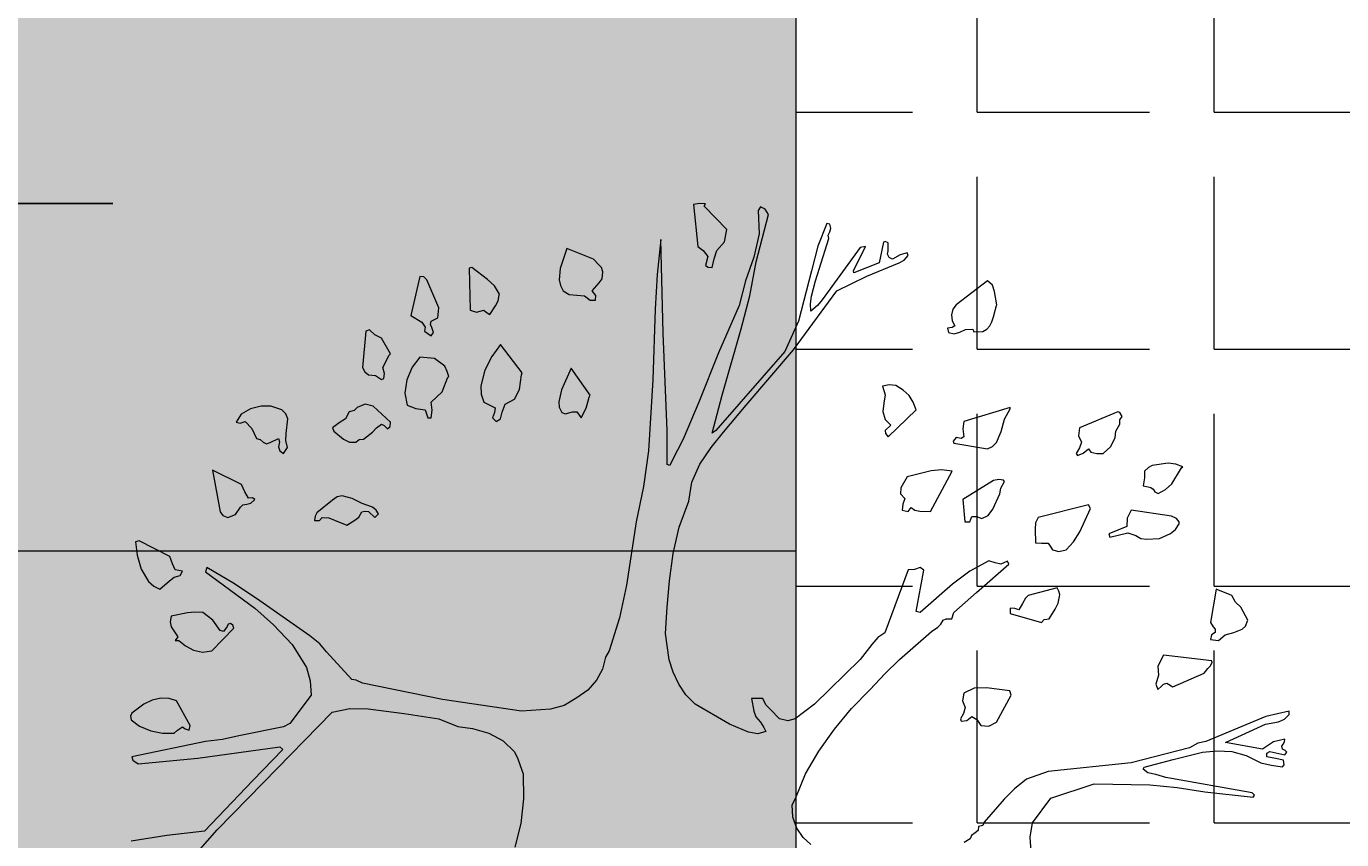
# Model space of a CAD drawing. Units: inches. Extents: x 84 to 1044, y -280 to 906.
# Tile 12 of 105: x 482 to 521, y -49 to -25. Entities that reach past the tile are written whole.
import ezdxf

# ---------------------------------------------------------------- set-up
doc = ezdxf.new("R2010")
doc.units = ezdxf.units.IN
for name, color, linetype, lineweight in [('A-ANNO-DIMS', 2, 'Continuous', 18), ('L-HRDS', 32, 'Continuous', 18), ('L-PLNT', 114, 'Continuous', 15)]:
    doc.layers.add(name, color=color, linetype=linetype, lineweight=lineweight)
doc.layers.add('L-HRDS-PATT', color=23, linetype='Continuous', lineweight=9, true_color=0xc2877b)
doc.layers.add('L-PLNT-PATT', color=9, linetype='Continuous', lineweight=9, true_color=0xafd9aa)
doc.styles.get("Standard").update_dxf_attribs({"font": 'arial.ttf'})
doc.dimstyles.get("Standard").update_dxf_attribs({"dimtxt": 0.18, "dimasz": 0.18, "dimexe": 0.18, "dimexo": 0.0625, "dimgap": 0.09, "dimtad": 0, "dimtih": 1, "dimtoh": 1, "dimdec": 4, "dimzin": 0, "dimdsep": 46, "dimtxsty": 'Standard', "dimcen": 0.09, "dimadec": 0, "dimazin": 0, "dimtfac": 1, "dimtdec": 4, "dimtofl": 0, "dimtmove": 0, "dimatfit": 3, "dimfxl": 1, "dimtolj": 1, "dimtzin": 0, "dimarcsym": 0})

# ---------------------------------------------------------------- blocks, each defined once
blk = doc.blocks.new('A$C37E508DF')
for p, q in [((0.6329, 1.5111), (0.6367, 1.5175)), ((0.6475, 1.4545), (0.6329, 1.5111)), ((0.6367, 1.5175), (0.6423, 1.5201)), ((0.6423, 1.5201), (0.6453, 1.5158)), ((0.6453, 1.5158), (0.644, 1.4879)), ((0.6826, 1.493), (0.7096, 1.5209)), ((0.7083, 1.5239), (0.7152, 1.5244)), ((0.7096, 1.5209), (0.7083, 1.5239)), ((0.7152, 1.5244), (0.7225, 1.5231)), ((0.7225, 1.5231), (0.7174, 1.4729)), ((0.5583, 1.4948), (0.5596, 1.4995)), ((0.5596, 1.4905), (0.5583, 1.4948)), ((0.5596, 1.4995), (0.563, 1.5003)), ((0.563, 1.5003), (0.5737, 1.4733)), ((0.4897, 1.4772), (0.4935, 1.4789)), ((0.4935, 1.4789), (0.4952, 1.478)), ((0.5613, 1.4862), (0.5596, 1.4905)), ((0.5608, 1.4823), (0.5613, 1.4862)), ((0.5767, 1.4317), (0.5608, 1.4823)), ((0.644, 1.4879), (0.6505, 1.46)), ((0.6852, 1.4785), (0.6826, 1.493)), ((0.6946, 1.4682), (0.6852, 1.4785)), ((0.7589, 1.3691), (0.7615, 1.481)), ((0.7615, 1.481), (0.7658, 1.4395)), ((0.4657, 1.4622), (0.4669, 1.4652)), ((0.4669, 1.4652), (0.4755, 1.463)), ((0.4755, 1.463), (0.4845, 1.4575)), ((0.4884, 1.4596), (0.4905, 1.4635)), ((0.4897, 1.4678), (0.4897, 1.4772)), ((0.4905, 1.4635), (0.4897, 1.4678)), ((0.4952, 1.478), (0.5004, 1.4532)), ((0.5313, 1.4437), (0.5167, 1.4729)), ((0.5167, 1.4729), (0.5231, 1.4716)), ((0.5231, 1.4716), (0.5686, 1.409)), ((0.5737, 1.4733), (0.5814, 1.4437)), ((0.6976, 1.4579), (0.6946, 1.4682)), ((0.7109, 1.4682), (0.7053, 1.4609)), ((0.7174, 1.4729), (0.7109, 1.4682)), ((0.8421, 1.4575), (0.8739, 1.4703)), ((0.8739, 1.4703), (0.882, 1.4463)), ((0.4708, 1.4566), (0.4657, 1.4622)), ((0.4764, 1.4532), (0.4708, 1.4566)), ((0.5154, 1.4373), (0.4764, 1.4532)), ((0.4845, 1.4575), (0.4884, 1.4596)), ((0.5004, 1.4532), (0.5308, 1.4412)), ((0.6552, 1.4137), (0.6475, 1.4545)), ((0.6505, 1.46), (0.6603, 1.4317)), ((0.7002, 1.4476), (0.6976, 1.4579)), ((0.7049, 1.448), (0.7002, 1.4476)), ((0.7083, 1.4502), (0.7049, 1.448)), ((0.7053, 1.4609), (0.7083, 1.4502)), ((0.831, 1.4424), (0.8323, 1.4476)), ((0.8323, 1.4476), (0.8357, 1.451)), ((0.8357, 1.451), (0.8421, 1.4575)), ((0.9686, 1.4334), (0.9875, 1.4476)), ((0.9875, 1.4476), (0.9905, 1.4467)), ((0.9905, 1.4467), (0.9896, 1.3966)), ((0.3649, 1.4266), (0.3709, 1.4317)), ((0.3709, 1.4317), (0.4086, 1.403)), ((0.551, 1.4197), (0.5154, 1.4373)), ((0.5308, 1.4412), (0.5313, 1.4437)), ((0.5814, 1.4133), (0.5767, 1.4317)), ((0.5814, 1.4437), (0.5969, 1.3833)), ((0.6603, 1.4317), (0.668, 1.4021)), ((0.7658, 1.4395), (0.7684, 1.3979)), ((0.8318, 1.4343), (0.831, 1.4424)), ((0.8353, 1.4292), (0.8318, 1.4343)), ((0.8829, 1.433), (0.8816, 1.4262)), ((0.882, 1.4463), (0.8829, 1.433)), ((0.9605, 1.4257), (0.9686, 1.4334)), ((1.0269, 1.3996), (1.0411, 1.433)), ((1.0411, 1.433), (1.045, 1.4365)), ((1.045, 1.4365), (1.0497, 1.4369)), ((1.0497, 1.4369), (1.0604, 1.3901)), ((0.3598, 1.403), (0.3628, 1.4189)), ((0.3628, 1.4189), (0.3649, 1.4266)), ((0.6029, 1.3494), (0.551, 1.4197)), ((0.8434, 1.4197), (0.8353, 1.4292)), ((0.8391, 1.4141), (0.8434, 1.4197)), ((0.8709, 1.4154), (0.8619, 1.4146)), ((0.8781, 1.4197), (0.8709, 1.4154)), ((0.8816, 1.4262), (0.8781, 1.4197)), ((0.9545, 1.4159), (0.9605, 1.4257)), ((0.9549, 1.4146), (0.9545, 1.4159)), ((0.3602, 1.4021), (0.3598, 1.403)), ((0.364, 1.3888), (0.3602, 1.4021)), ((0.4086, 1.403), (0.4125, 1.3979)), ((0.5686, 1.409), (0.5741, 1.4021)), ((0.5741, 1.4021), (0.5823, 1.3953)), ((0.5827, 1.4043), (0.5814, 1.4133)), ((0.5823, 1.3953), (0.5827, 1.4043)), ((0.6655, 1.3743), (0.6552, 1.4137)), ((0.668, 1.4021), (0.6925, 1.3455)), ((0.8395, 1.4086), (0.8391, 1.4141)), ((0.846, 1.4086), (0.8395, 1.4086)), ((0.8528, 1.4137), (0.846, 1.4086)), ((0.8619, 1.4146), (0.8528, 1.4137)), ((0.9558, 1.4077), (0.9549, 1.4146)), ((0.9592, 1.4017), (0.9558, 1.4077)), ((0.966, 1.3914), (0.9592, 1.4017)), ((1.0282, 1.3876), (1.0269, 1.3996)), ((0.3657, 1.3828), (0.364, 1.3888)), ((0.4125, 1.3979), (0.4142, 1.391)), ((0.4142, 1.391), (0.4134, 1.3837)), ((0.7684, 1.3979), (0.771, 1.3134)), ((0.9703, 1.3944), (0.966, 1.3914)), ((0.9733, 1.3966), (0.9703, 1.3944)), ((0.9819, 1.3944), (0.9733, 1.3966)), ((0.9896, 1.3966), (0.9819, 1.3944)), ((1.0359, 1.3833), (1.0282, 1.3876)), ((1.0604, 1.3901), (1.0471, 1.3824)), ((0.3683, 1.3781), (0.3657, 1.3828)), ((0.3718, 1.3738), (0.3683, 1.3781)), ((0.3765, 1.3713), (0.3718, 1.3738)), ((0.3872, 1.3708), (0.3765, 1.3713)), ((0.3885, 1.3738), (0.3872, 1.3708)), ((0.3971, 1.3734), (0.3885, 1.3738)), ((0.4039, 1.3704), (0.3971, 1.3734)), ((0.4108, 1.3683), (0.4039, 1.3704)), ((0.4134, 1.3837), (0.4099, 1.3781)), ((0.4099, 1.3781), (0.4134, 1.376)), ((0.4176, 1.37), (0.4108, 1.3683)), ((0.4134, 1.376), (0.4189, 1.3751)), ((0.4189, 1.3751), (0.4176, 1.37)), ((0.5969, 1.3833), (0.6132, 1.3472)), ((0.6882, 1.2949), (0.6655, 1.3743)), ((0.7538, 1.2529), (0.7589, 1.3691)), ((1.0334, 1.37), (1.0351, 1.376)), ((1.0359, 1.3661), (1.0334, 1.37)), ((1.0351, 1.376), (1.0368, 1.3794)), ((1.0368, 1.3794), (1.0359, 1.3833)), ((1.0441, 1.3717), (1.0359, 1.3661)), ((1.0471, 1.3824), (1.0432, 1.3764)), ((1.0432, 1.3764), (1.0441, 1.3717)), ((1.1033, 1.367), (1.1097, 1.373)), ((1.1097, 1.373), (1.114, 1.3717)), ((1.114, 1.3717), (1.1183, 1.328)), ((0.9274, 1.3215), (0.9532, 1.3554)), ((0.9532, 1.3554), (0.9635, 1.3413)), ((1.0848, 1.3443), (1.0955, 1.3631)), ((1.0955, 1.3631), (1.1033, 1.367)), ((0.6595, 1.2829), (0.6029, 1.3494)), ((0.6132, 1.3472), (0.6959, 1.2529)), ((0.6925, 1.3455), (0.7161, 1.2868)), ((0.9635, 1.3413), (0.9721, 1.325)), ((1.0197, 1.3297), (1.0321, 1.3387)), ((1.0321, 1.3387), (1.0497, 1.3404)), ((1.0497, 1.3404), (1.0587, 1.3284)), ((1.0861, 1.343), (1.0848, 1.3443)), ((1.0938, 1.328), (1.0861, 1.343)), ((0.846, 1.2949), (0.8687, 1.3271)), ((0.8687, 1.3271), (0.8803, 1.3014)), ((0.9279, 1.3194), (0.9274, 1.3215)), ((0.9721, 1.325), (0.9768, 1.3061)), ((1.0149, 1.3172), (1.0171, 1.3232)), ((1.0171, 1.3232), (1.0197, 1.3297)), ((1.0587, 1.3284), (1.0651, 1.3134)), ((1.0917, 1.3207), (1.0938, 1.328)), ((1.1153, 1.3228), (1.111, 1.3194)), ((1.1183, 1.328), (1.1153, 1.3228)), ((0.4717, 1.3009), (0.4807, 1.3065)), ((0.4807, 1.3065), (0.4884, 1.3074)), ((0.4884, 1.3074), (0.4965, 1.3057)), ((0.4965, 1.3057), (0.4935, 1.2954)), ((0.771, 1.3134), (0.7761, 1.2285)), ((0.9305, 1.3018), (0.9279, 1.3194)), ((0.9768, 1.3061), (0.9763, 1.2962)), ((1.0162, 1.3164), (1.0149, 1.3172)), ((1.0231, 1.2988), (1.0162, 1.3164)), ((1.0651, 1.3134), (1.0677, 1.2975)), ((1.0925, 1.3151), (1.0917, 1.3207)), ((1.0955, 1.3138), (1.0925, 1.3151)), ((1.1028, 1.3185), (1.0955, 1.3138)), ((1.111, 1.3194), (1.1028, 1.3185)), ((0.4597, 1.2868), (0.4648, 1.2945)), ((0.4648, 1.2945), (0.4717, 1.3009)), ((0.4935, 1.2954), (0.4948, 1.2855)), ((0.7002, 1.2495), (0.6882, 1.2949)), ((0.8473, 1.2924), (0.846, 1.2949)), ((0.8507, 1.2795), (0.8473, 1.2924)), ((0.8803, 1.3014), (0.8833, 1.2872)), ((0.9365, 1.2902), (0.9305, 1.3018)), ((0.9476, 1.2842), (0.9365, 1.2902)), ((0.9763, 1.2962), (0.9733, 1.2868)), ((1.0359, 1.2868), (1.0231, 1.2988)), ((1.0677, 1.2975), (1.0647, 1.2829)), ((0.2101, 1.2696), (0.2127, 1.2744)), ((0.2127, 1.2744), (0.2152, 1.2752)), ((0.2152, 1.2752), (0.2611, 1.2559)), ((0.3439, 1.2804), (0.3992, 1.2636)), ((0.3439, 1.2787), (0.3439, 1.2804)), ((0.3507, 1.2662), (0.3439, 1.2787)), ((0.4562, 1.2774), (0.4597, 1.2868)), ((0.4897, 1.2452), (0.4562, 1.2774)), ((0.4961, 1.2756), (0.4935, 1.2658)), ((0.4948, 1.2855), (0.4961, 1.2756)), ((0.6865, 1.2508), (0.6595, 1.2829)), ((0.7161, 1.2868), (0.7349, 1.2422)), ((0.8567, 1.2679), (0.8507, 1.2795)), ((0.8619, 1.2752), (0.8567, 1.2679)), ((0.867, 1.2752), (0.8619, 1.2752)), ((0.8713, 1.2739), (0.867, 1.2752)), ((0.8756, 1.2726), (0.8713, 1.2739)), ((0.8799, 1.2744), (0.8756, 1.2726)), ((0.8829, 1.2808), (0.8799, 1.2744)), ((0.8833, 1.2872), (0.8829, 1.2808)), ((0.951, 1.2748), (0.9476, 1.2842)), ((0.9532, 1.2666), (0.951, 1.2748)), ((0.9733, 1.2868), (0.9596, 1.2799)), ((0.9596, 1.2799), (0.9605, 1.2744)), ((0.9605, 1.2744), (0.9626, 1.2679)), ((1.0347, 1.2769), (1.0359, 1.2868)), ((1.0359, 1.2679), (1.0347, 1.2769)), ((1.0432, 1.2774), (1.0402, 1.2679)), ((1.0544, 1.2791), (1.0432, 1.2774)), ((1.0647, 1.2829), (1.0544, 1.2791)), ((1.0848, 1.2628), (1.1054, 1.2817)), ((1.1054, 1.2817), (1.1148, 1.2842)), ((1.1148, 1.2842), (1.1247, 1.2804)), ((1.1247, 1.2804), (1.1281, 1.2765)), ((1.1281, 1.2765), (1.1341, 1.2752)), ((1.1341, 1.2752), (1.1384, 1.2666)), ((1.21, 1.2726), (1.2147, 1.2774)), ((1.2147, 1.2774), (1.2276, 1.2817)), ((1.2276, 1.2817), (1.2392, 1.2817)), ((1.2392, 1.2817), (1.2521, 1.2787)), ((1.2521, 1.2787), (1.2632, 1.2722)), ((0.2127, 1.2654), (0.2101, 1.2696)), ((0.2127, 1.2602), (0.2127, 1.2654)), ((0.2174, 1.2521), (0.2127, 1.2602)), ((0.3546, 1.2516), (0.3507, 1.2662)), ((0.3992, 1.2636), (0.4005, 1.2546)), ((0.4935, 1.2658), (0.4867, 1.2589)), ((0.4867, 1.2589), (0.4935, 1.2529)), ((0.9583, 1.2636), (0.9532, 1.2666)), ((0.9626, 1.2679), (0.9583, 1.2636)), ((1.0402, 1.2679), (1.0359, 1.2679)), ((1.0852, 1.2576), (1.0848, 1.2628)), ((1.0921, 1.2585), (1.0883, 1.2546)), ((1.0955, 1.2602), (1.0921, 1.2585)), ((1.1015, 1.2559), (1.0955, 1.2602)), ((1.1384, 1.2666), (1.1461, 1.2619)), ((1.1461, 1.2619), (1.1539, 1.2559)), ((1.2075, 1.2666), (1.21, 1.2726)), ((1.2096, 1.2491), (1.2075, 1.2666)), ((1.2585, 1.2636), (1.2503, 1.2551)), ((1.2645, 1.2615), (1.2585, 1.2636)), ((1.2632, 1.2722), (1.2692, 1.2628)), ((1.2692, 1.2628), (1.2645, 1.2615)), ((0.2182, 1.2443), (0.2174, 1.2521)), ((0.2234, 1.2336), (0.2182, 1.2443)), ((0.262, 1.2465), (0.2586, 1.2388)), ((0.2611, 1.2559), (0.262, 1.2465)), ((0.3602, 1.2383), (0.3546, 1.2516)), ((0.4005, 1.2546), (0.3992, 1.2452)), ((0.3992, 1.2452), (0.4026, 1.2431)), ((0.4026, 1.2431), (0.4086, 1.2443)), ((0.4086, 1.2443), (0.4121, 1.2401)), ((0.4931, 1.2491), (0.4897, 1.2452)), ((0.4935, 1.2529), (0.4931, 1.2491)), ((0.7015, 1.2323), (0.6865, 1.2508)), ((0.6959, 1.2529), (0.7002, 1.2495)), ((0.7538, 1.2122), (0.7538, 1.2529)), ((1.0883, 1.2546), (1.0852, 1.2576)), ((1.1063, 1.2508), (1.1015, 1.2559)), ((1.117, 1.2422), (1.1063, 1.2508)), ((1.1526, 1.2521), (1.141, 1.2422)), ((1.1539, 1.2559), (1.1526, 1.2521)), ((1.21, 1.2409), (1.2096, 1.2491)), ((1.2186, 1.2431), (1.2173, 1.2392)), ((1.2285, 1.2383), (1.2186, 1.2431)), ((1.2448, 1.2431), (1.2405, 1.2418)), ((1.2503, 1.2551), (1.2448, 1.2431)), ((0.2328, 1.2251), (0.2234, 1.2336)), ((0.2474, 1.2268), (0.2401, 1.2251)), ((0.2504, 1.2306), (0.2474, 1.2268)), ((0.2568, 1.2255), (0.2504, 1.2306)), ((0.2586, 1.2388), (0.2611, 1.2319)), ((0.2611, 1.2319), (0.265, 1.2251)), ((0.3649, 1.2336), (0.3602, 1.2383)), ((0.3709, 1.2306), (0.3649, 1.2336)), ((0.4112, 1.2375), (0.3709, 1.2306)), ((0.4121, 1.2401), (0.4112, 1.2375)), ((0.7148, 1.2126), (0.7015, 1.2323)), ((0.7349, 1.2422), (0.7482, 1.216)), ((0.7761, 1.2285), (0.7821, 1.1856)), ((1.1221, 1.2418), (1.117, 1.2422)), ((1.126, 1.2388), (1.1221, 1.2418)), ((1.1337, 1.2388), (1.126, 1.2388)), ((1.141, 1.2422), (1.1337, 1.2388)), ((1.2079, 1.2323), (1.21, 1.2409)), ((1.2126, 1.2251), (1.2079, 1.2323)), ((1.2169, 1.2285), (1.2126, 1.2251)), ((1.2186, 1.2332), (1.2169, 1.2285)), ((1.2173, 1.2392), (1.2186, 1.2332)), ((1.2328, 1.2366), (1.2285, 1.2383)), ((1.2371, 1.2388), (1.2328, 1.2366)), ((1.2405, 1.2418), (1.2371, 1.2388)), ((0.1376, 1.2092), (0.1458, 1.2126)), ((0.1458, 1.2126), (0.1548, 1.2135)), ((0.1548, 1.2135), (0.1741, 1.2109)), ((0.1741, 1.2109), (0.1784, 1.2083)), ((0.2401, 1.2251), (0.2328, 1.2251)), ((0.2633, 1.2229), (0.2568, 1.2255)), ((0.265, 1.2251), (0.2633, 1.2229)), ((0.7246, 1.1908), (0.7148, 1.2126)), ((0.7482, 1.216), (0.7508, 1.2109)), ((0.7508, 1.2109), (0.7538, 1.2122)), ((0.1389, 1.2079), (0.1376, 1.2092)), ((0.1505, 1.189), (0.1389, 1.2079)), ((0.1784, 1.2083), (0.1831, 1.204)), ((0.1831, 1.204), (0.1831, 1.1959)), ((0.1831, 1.1959), (0.1848, 1.1865)), ((0.4134, 1.204), (0.4258, 1.2058)), ((0.4391, 1.156), (0.4134, 1.204)), ((0.4258, 1.2058), (0.4382, 1.2045)), ((0.4382, 1.2045), (0.4669, 1.1972)), ((0.4669, 1.1972), (0.4747, 1.1843)), ((1.2628, 1.1882), (1.2975, 1.2053)), ((1.2975, 1.2053), (1.2885, 1.1556)), ((0.1582, 1.1822), (0.1505, 1.189)), ((0.1668, 1.1775), (0.1582, 1.1822)), ((0.1728, 1.1826), (0.1711, 1.1792)), ((0.1758, 1.1847), (0.1728, 1.1826)), ((0.1788, 1.1852), (0.1758, 1.1847)), ((0.1848, 1.1865), (0.1788, 1.1852)), ((0.3507, 1.1916), (0.352, 1.1933)), ((0.355, 1.1839), (0.3507, 1.1916)), ((0.352, 1.1933), (0.3576, 1.1942)), ((0.3563, 1.177), (0.355, 1.1839)), ((0.3576, 1.1942), (0.364, 1.1929)), ((0.364, 1.1929), (0.4005, 1.1702)), ((0.4747, 1.1843), (0.4751, 1.177)), ((0.7281, 1.168), (0.7246, 1.1908)), ((0.7821, 1.1856), (0.7911, 1.1436)), ((1.2589, 1.1792), (1.2628, 1.1882)), ((0.1711, 1.1792), (0.1668, 1.1775)), ((0.2478, 1.1594), (0.2504, 1.1637)), ((0.2504, 1.1637), (0.3104, 1.1487)), ((0.3645, 1.1586), (0.3563, 1.177)), ((0.4005, 1.1702), (0.3979, 1.1436)), ((0.4751, 1.177), (0.47, 1.1714)), ((0.47, 1.1714), (0.4721, 1.1646)), ((0.4721, 1.1646), (0.473, 1.1573)), ((0.7396, 1.1371), (0.7281, 1.168)), ((1.1063, 1.1612), (1.1187, 1.1655)), ((1.1187, 1.1655), (1.1307, 1.1714)), ((1.1307, 1.1714), (1.1423, 1.1744)), ((1.1423, 1.1744), (1.1483, 1.1732)), ((1.1483, 1.1732), (1.1539, 1.1693)), ((1.1539, 1.1693), (1.1727, 1.1543)), ((1.2469, 1.1702), (1.2495, 1.1723)), ((1.2478, 1.1693), (1.2469, 1.1702)), ((1.2516, 1.1659), (1.2478, 1.1693)), ((1.2495, 1.1723), (1.2546, 1.1719)), ((1.2563, 1.1646), (1.2516, 1.1659)), ((1.2546, 1.1719), (1.2589, 1.1792)), ((1.2611, 1.1637), (1.2563, 1.1646)), ((1.2641, 1.1612), (1.2611, 1.1637)), ((0.1449, 1.1474), (0.1509, 1.1504)), ((0.1509, 1.1504), (0.1994, 1.1573)), ((0.1994, 1.1573), (0.2041, 1.1479)), ((0.2607, 1.1316), (0.2478, 1.1594)), ((0.3104, 1.1487), (0.3134, 1.1423)), ((0.37, 1.1509), (0.3645, 1.1586)), ((0.3778, 1.1474), (0.37, 1.1509)), ((0.3842, 1.15), (0.3778, 1.1474)), ((0.3898, 1.15), (0.3842, 1.15)), ((0.3923, 1.1436), (0.3898, 1.15)), ((0.4519, 1.1564), (0.4391, 1.156)), ((0.458, 1.1573), (0.4519, 1.1564)), ((0.4622, 1.1607), (0.458, 1.1573)), ((0.4657, 1.156), (0.4622, 1.1607)), ((0.473, 1.1573), (0.4657, 1.156)), ((1.099, 1.153), (1.102, 1.1573)), ((1.1033, 1.1487), (1.099, 1.153)), ((1.102, 1.1573), (1.1063, 1.1612)), ((1.111, 1.156), (1.1033, 1.1487)), ((1.1153, 1.1564), (1.111, 1.156)), ((1.1191, 1.1556), (1.1153, 1.1564)), ((1.1226, 1.1492), (1.1191, 1.1556)), ((1.1273, 1.1453), (1.1226, 1.1492)), ((1.1586, 1.1483), (1.1517, 1.1453)), ((1.1663, 1.1487), (1.1586, 1.1483)), ((1.1697, 1.1449), (1.1663, 1.1487)), ((1.1727, 1.1543), (1.1749, 1.1504)), ((1.1749, 1.1504), (1.1757, 1.1449)), ((1.2701, 1.1522), (1.2641, 1.1612)), ((1.2791, 1.1487), (1.2701, 1.1522)), ((1.2851, 1.1509), (1.2791, 1.1487)), ((1.2885, 1.1556), (1.2851, 1.1509)), ((0.1419, 1.1436), (0.1449, 1.1474)), ((0.1419, 1.141), (0.1419, 1.1436)), ((0.1462, 1.1342), (0.1419, 1.141)), ((0.1522, 1.1294), (0.1462, 1.1342)), ((0.2041, 1.1479), (0.2045, 1.138)), ((0.2045, 1.138), (0.226, 1.129)), ((0.3134, 1.1423), (0.3139, 1.1346)), ((0.3139, 1.1346), (0.3134, 1.1183)), ((0.3979, 1.1436), (0.3923, 1.1436)), ((0.7469, 1.1054), (0.7396, 1.1371)), ((0.7911, 1.1436), (0.8027, 1.0677)), ((1.1367, 1.1393), (1.1273, 1.1453)), ((1.1517, 1.1453), (1.1367, 1.1393)), ((1.1757, 1.1449), (1.1697, 1.1449)), ((0.1655, 1.1234), (0.1522, 1.1294)), ((0.181, 1.1226), (0.1655, 1.1234)), ((0.1878, 1.1234), (0.181, 1.1226)), ((0.1938, 1.1273), (0.1878, 1.1234)), ((0.2032, 1.1303), (0.1938, 1.1273)), ((0.2247, 1.1251), (0.2032, 1.1303)), ((0.226, 1.129), (0.2247, 1.1251)), ((0.268, 1.1196), (0.2607, 1.1316)), ((0.277, 1.1101), (0.268, 1.1196)), ((0.2984, 1.1179), (0.2959, 1.1144)), ((0.3066, 1.1179), (0.2984, 1.1179)), ((0.3134, 1.1183), (0.3066, 1.1179)), ((1.3485, 1.102), (1.385, 1.1209)), ((1.385, 1.1209), (1.3897, 1.1196)), ((1.3897, 1.1196), (1.3875, 1.1037)), ((0.2856, 1.108), (0.277, 1.1101)), ((0.2933, 1.1101), (0.2856, 1.108)), ((0.2959, 1.1144), (0.2933, 1.1101)), ((0.7512, 1.0728), (0.7469, 1.1054)), ((1.3455, 1.0934), (1.3485, 1.102)), ((1.3875, 1.1037), (1.3828, 1.087)), ((0.3456, 1.093), (0.3469, 1.0964)), ((0.3842, 1.0591), (0.3456, 1.093)), ((0.3469, 1.0964), (0.355, 1.093)), ((0.355, 1.093), (0.3619, 1.0943)), ((0.3619, 1.0943), (0.3692, 1.0968)), ((0.3692, 1.0968), (0.3923, 1.0844)), ((0.4472, 1.0857), (0.4515, 1.0887)), ((0.4562, 1.0364), (0.4472, 1.0857)), ((0.4515, 1.0887), (0.4584, 1.0865)), ((0.4584, 1.0865), (0.4657, 1.0861)), ((0.4657, 1.0861), (0.4939, 1.0107)), ((1.2713, 1.0694), (1.3044, 1.0887)), ((1.3044, 1.0887), (1.3057, 1.0835)), ((1.3335, 1.0844), (1.3421, 1.0861)), ((1.3421, 1.0861), (1.3455, 1.0934)), ((1.3828, 1.087), (1.3738, 1.072)), ((0.3923, 1.0844), (0.4129, 1.069)), ((0.7538, 1.0415), (0.7512, 1.0728)), ((1.2409, 1.0488), (1.2713, 1.0694)), ((1.3057, 1.0835), (1.2469, 1.0402)), ((1.3361, 1.0793), (1.3335, 1.0844)), ((1.3434, 1.0771), (1.3361, 1.0793)), ((1.349, 1.0728), (1.3434, 1.0771)), ((1.3605, 1.063), (1.349, 1.0728)), ((1.3738, 1.072), (1.3678, 1.0664)), ((0.0746, 1.0475), (0.0789, 1.0552)), ((0.0789, 1.0552), (0.0978, 1.063)), ((0.0978, 1.063), (0.1042, 1.0231)), ((0.2847, 1.0565), (0.2856, 1.0604)), ((0.2851, 1.054), (0.2847, 1.0565)), ((0.2864, 1.0463), (0.2851, 1.054)), ((0.2856, 1.0604), (0.2877, 1.0647)), ((0.2877, 1.0647), (0.3224, 1.0552)), ((0.3224, 1.0552), (0.3255, 1.0522)), ((0.4112, 1.0351), (0.3842, 1.0591)), ((0.4129, 1.069), (0.4515, 1.0351)), ((0.8027, 1.0677), (0.8108, 1.0287)), ((1.3678, 1.0664), (1.3605, 1.063)), ((0.0596, 1.0257), (0.0682, 1.0415)), ((0.0682, 1.0415), (0.0746, 1.0475)), ((0.2899, 1.039), (0.2864, 1.0463)), ((0.2972, 1.0274), (0.2899, 1.039)), ((0.3255, 1.0522), (0.3293, 1.0458)), ((0.3293, 1.0458), (0.3336, 1.0381)), ((0.3336, 1.0381), (0.3383, 1.0398)), ((0.3383, 1.0398), (0.3439, 1.0402)), ((0.3439, 1.0402), (0.3439, 1.0338)), ((0.7559, 1.0098), (0.7538, 1.0415)), ((1.1813, 1.0072), (1.2409, 1.0488)), ((1.2469, 1.0402), (1.2246, 1.0201)), ((0.0626, 1.0188), (0.0596, 1.0257)), ((0.1042, 1.0231), (0.1012, 1.018)), ((0.3032, 1.0265), (0.2972, 1.0274)), ((0.3066, 1.0231), (0.3032, 1.0265)), ((0.3439, 1.0338), (0.3066, 1.0231)), ((0.4138, 1.0274), (0.4112, 1.0351)), ((0.4202, 1.0274), (0.4138, 1.0274)), ((0.4241, 1.0257), (0.4202, 1.0274)), ((0.4267, 1.0209), (0.4241, 1.0257)), ((0.4515, 1.0351), (0.4562, 1.0364)), ((0.8108, 1.0287), (0.8233, 0.9892)), ((1.2885, 1.0136), (1.2971, 1.0257)), ((1.2971, 1.0257), (1.3091, 1.0351)), ((1.3091, 1.0351), (1.3185, 1.0355)), ((1.3185, 1.0355), (1.3275, 1.0347)), ((1.3275, 1.0347), (1.3468, 1.0308)), ((1.3468, 1.0308), (1.3481, 1.0239)), ((1.3481, 1.0239), (1.3468, 1.018)), ((0.0665, 1.0149), (0.0626, 1.0188)), ((0.0763, 1.0111), (0.0665, 1.0149)), ((0.087, 1.0085), (0.0763, 1.0111)), ((0.0948, 1.0016), (0.087, 1.0085)), ((0.1012, 1.018), (0.099, 1.0149)), ((0.099, 1.0149), (0.099, 1.0111)), ((0.099, 1.0111), (0.1033, 1.0085)), ((0.1033, 1.0085), (0.1042, 1.0029)), ((0.4305, 1.0175), (0.4267, 1.0209)), ((0.4378, 1.0124), (0.4305, 1.0175)), ((0.476, 0.9789), (0.4378, 1.0124)), ((0.4939, 1.0107), (0.5021, 1.0051)), ((0.7516, 0.9785), (0.7559, 1.0098)), ((1.1693, 0.9974), (1.1813, 1.0072)), ((1.2246, 1.0201), (1.2023, 0.9969)), ((1.2718, 1.0162), (1.2731, 1.0197)), ((1.2984, 0.9892), (1.2718, 1.0162)), ((1.2731, 1.0197), (1.2761, 1.0218)), ((1.2761, 1.0218), (1.2786, 1.0209)), ((1.2786, 1.0209), (1.2799, 1.0184)), ((1.2799, 1.0184), (1.2842, 1.0124)), ((1.2842, 1.0124), (1.2885, 1.0136)), ((1.3468, 1.018), (1.3391, 1.0059)), ((0.1042, 1.0029), (0.0948, 1.0016)), ((0.5021, 1.0051), (0.5094, 0.9969)), ((0.5094, 0.9969), (0.5231, 0.9789)), ((1.1612, 0.9879), (1.1693, 0.9974)), ((1.2023, 0.9969), (1.1852, 0.9691)), ((1.3297, 0.9952), (1.3202, 0.9901)), ((1.3378, 1.0016), (1.3297, 0.9952)), ((1.3421, 1.0016), (1.3378, 1.0016)), ((1.3391, 1.0059), (1.3421, 1.0016)), ((0.1025, 0.9751), (0.1029, 0.9772)), ((0.1046, 0.9708), (0.1025, 0.9751)), ((0.1029, 0.9772), (0.1604, 0.9841)), ((0.1604, 0.9841), (0.1672, 0.9708)), ((0.4939, 0.9618), (0.476, 0.9789)), ((0.5231, 0.9789), (0.578, 0.9253)), ((0.7469, 0.9635), (0.7516, 0.9785)), ((0.8233, 0.9892), (0.8275, 0.9815)), ((0.8275, 0.9815), (0.8314, 0.9673)), ((1.1311, 0.9549), (1.1612, 0.9879)), ((1.3095, 0.9875), (1.2984, 0.9892)), ((1.3202, 0.9901), (1.3095, 0.9875)), ((0.1076, 0.9682), (0.1046, 0.9708)), ((0.1119, 0.9626), (0.1076, 0.9682)), ((0.1496, 0.9463), (0.1119, 0.9626)), ((0.1672, 0.9708), (0.1664, 0.9601)), ((0.1664, 0.9601), (0.1698, 0.9493)), ((0.5111, 0.9429), (0.4939, 0.9618)), ((0.7401, 0.9493), (0.7469, 0.9635)), ((0.8314, 0.9673), (0.8383, 0.954)), ((1.1852, 0.9691), (1.1809, 0.9532)), ((0.1565, 0.9506), (0.1496, 0.9463)), ((0.1604, 0.9493), (0.1565, 0.9506)), ((0.1629, 0.9468), (0.1604, 0.9493)), ((0.1672, 0.9429), (0.1629, 0.9468)), ((0.1698, 0.9493), (0.1672, 0.9429)), ((0.3443, 0.9412), (0.3722, 0.9451)), ((0.3722, 0.9451), (0.3868, 0.9446)), ((0.3868, 0.9446), (0.3992, 0.9386)), ((0.7315, 0.9365), (0.7401, 0.9493)), ((0.8383, 0.954), (0.8486, 0.942)), ((1.0227, 0.9309), (1.1183, 0.9506)), ((1.1183, 0.9506), (1.1256, 0.954)), ((1.1256, 0.954), (1.1311, 0.9549)), ((1.1809, 0.9532), (1.1796, 0.936)), ((0.3426, 0.936), (0.3443, 0.9412)), ((0.3602, 0.9039), (0.3426, 0.936)), ((0.4009, 0.9292), (0.3975, 0.9215)), ((0.3992, 0.9386), (0.4009, 0.9292)), ((0.5334, 0.9202), (0.5111, 0.9429)), ((0.6359, 0.9245), (0.6397, 0.9322)), ((0.6397, 0.9322), (0.653, 0.9322)), ((0.653, 0.9322), (0.6505, 0.9172)), ((0.7203, 0.9253), (0.7315, 0.9365)), ((0.8486, 0.942), (0.8619, 0.933)), ((0.8619, 0.933), (0.8769, 0.9236)), ((0.9279, 0.9172), (1.0227, 0.9309)), ((1.1796, 0.936), (1.2049, 0.9022)), ((1.3241, 0.9), (1.3404, 0.9292)), ((1.3404, 0.9292), (1.3494, 0.9322)), ((1.3494, 0.9322), (1.3592, 0.9326)), ((1.3592, 0.9326), (1.3695, 0.93)), ((1.3695, 0.93), (1.3794, 0.9253)), ((0.0103, 0.9129), (0.0103, 0.9172)), ((0.0103, 0.9172), (0.0382, 0.9107)), ((0.0159, 0.9073), (0.0103, 0.9129)), ((0.3975, 0.9215), (0.3996, 0.9142)), ((0.3996, 0.9142), (0.4031, 0.9077)), ((0.554, 0.8953), (0.5334, 0.9202)), ((0.578, 0.9253), (0.6011, 0.9077)), ((0.6196, 0.9077), (0.6303, 0.9189)), ((0.6303, 0.9189), (0.6359, 0.9245)), ((0.6505, 0.9172), (0.6479, 0.9103)), ((0.6796, 0.9013), (0.7203, 0.9253)), ((0.8769, 0.9236), (0.8936, 0.9193)), ((0.8936, 0.9193), (0.9279, 0.9172)), ((1.0685, 0.9142), (1.0269, 0.9077)), ((1.1114, 0.9198), (1.0685, 0.9142)), ((1.1333, 0.9202), (1.1114, 0.9198)), ((1.1543, 0.9159), (1.1333, 0.9202)), ((1.2371, 0.8314), (1.1543, 0.9159)), ((1.3794, 0.9253), (1.394, 0.9146)), ((1.394, 0.9146), (1.3957, 0.9112)), ((0.0232, 0.9043), (0.0159, 0.9073)), ((0.0386, 0.9013), (0.0232, 0.9043)), ((0.0382, 0.9107), (0.1098, 0.8807)), ((0.0866, 0.8794), (0.0386, 0.9013)), ((0.3692, 0.8992), (0.3602, 0.9039)), ((0.379, 0.9), (0.3692, 0.8992)), ((0.3838, 0.9069), (0.379, 0.9)), ((0.3898, 0.9107), (0.3838, 0.9069)), ((0.3958, 0.906), (0.3898, 0.9107)), ((0.4026, 0.9052), (0.3958, 0.906)), ((0.4031, 0.9077), (0.4026, 0.9052)), ((0.6011, 0.9077), (0.6097, 0.9056)), ((0.6097, 0.9056), (0.6196, 0.9077)), ((0.6384, 0.8974), (0.6359, 0.8927)), ((0.6423, 0.9039), (0.6384, 0.8974)), ((0.6479, 0.9103), (0.6423, 0.9039)), ((0.6569, 0.8919), (0.6796, 0.9013)), ((1.0042, 0.8987), (0.9866, 0.8962)), ((1.0269, 0.9077), (1.0042, 0.8987)), ((1.2049, 0.9022), (1.2126, 0.8983)), ((1.2126, 0.8983), (1.2662, 0.8876)), ((1.3254, 0.8944), (1.3241, 0.9)), ((1.3335, 0.8983), (1.3301, 0.8957)), ((1.3395, 0.8944), (1.3335, 0.8983)), ((1.3846, 0.8992), (1.3713, 0.8936)), ((1.3948, 0.9065), (1.3846, 0.8992)), ((1.3957, 0.9112), (1.3948, 0.9065)), ((0.0159, 0.8803), (0.0154, 0.8837)), ((0.0154, 0.8837), (0.0292, 0.8803)), ((0.1098, 0.8807), (0.1196, 0.8786)), ((0.5728, 0.8691), (0.554, 0.8953)), ((0.6359, 0.8927), (0.6457, 0.8897)), ((0.6457, 0.8897), (0.6569, 0.8919)), ((0.9498, 0.8816), (0.9369, 0.8687)), ((0.9673, 0.8906), (0.9498, 0.8816)), ((0.9866, 0.8962), (0.9673, 0.8906)), ((1.2662, 0.8876), (1.2855, 0.8833)), ((1.2855, 0.8833), (1.3057, 0.8807)), ((1.3057, 0.8807), (1.394, 0.8623)), ((1.3301, 0.8957), (1.3254, 0.8944)), ((1.3434, 0.8906), (1.3395, 0.8944)), ((1.3571, 0.8906), (1.3434, 0.8906)), ((1.3713, 0.8936), (1.3571, 0.8906)), ((0.0133, 0.8679), (0.015, 0.87)), ((0.0154, 0.8649), (0.0133, 0.8679)), ((0.015, 0.87), (0.0184, 0.8717)), ((0.0334, 0.8687), (0.0154, 0.8649)), ((0.0176, 0.8777), (0.0159, 0.8803)), ((0.0193, 0.8752), (0.0176, 0.8777)), ((0.0184, 0.8717), (0.0193, 0.8752)), ((0.0292, 0.8803), (0.0424, 0.8717)), ((0.0369, 0.8666), (0.0334, 0.8687)), ((0.0369, 0.8623), (0.0369, 0.8666)), ((0.0424, 0.8717), (0.0866, 0.8794)), ((0.0789, 0.8687), (0.0617, 0.864)), ((0.0965, 0.8696), (0.0789, 0.8687)), ((0.1141, 0.8679), (0.0965, 0.8696)), ((0.1492, 0.8593), (0.1141, 0.8679)), ((0.1196, 0.8786), (0.1295, 0.873)), ((0.1295, 0.873), (0.1994, 0.8554)), ((0.5887, 0.8421), (0.5728, 0.8691)), ((0.9369, 0.8687), (0.933, 0.861)), ((1.2169, 0.8743), (1.2135, 0.8713)), ((1.2135, 0.8713), (1.2491, 0.834)), ((1.3151, 0.8606), (1.2169, 0.8743)), ((0.0163, 0.8529), (0.0171, 0.8584)), ((0.0184, 0.8503), (0.0163, 0.8529)), ((0.0171, 0.8584), (0.0266, 0.8602)), ((0.0317, 0.8524), (0.0184, 0.8503)), ((0.0266, 0.8602), (0.0369, 0.8623)), ((0.0442, 0.8554), (0.0317, 0.8524)), ((0.0617, 0.864), (0.0442, 0.8554)), ((0.1835, 0.8499), (0.1492, 0.8593)), ((0.1848, 0.8477), (0.1835, 0.8499)), ((0.1994, 0.8554), (0.2984, 0.8447)), ((0.9296, 0.852), (0.9262, 0.8421)), ((0.933, 0.861), (0.9296, 0.852)), ((1.3863, 0.8541), (1.3151, 0.8606)), ((1.3927, 0.8584), (1.3863, 0.8541)), ((1.394, 0.8623), (1.3927, 0.8584)), ((0.0545, 0.8194), (0.1578, 0.8378)), ((0.1578, 0.8378), (0.1698, 0.8413)), ((0.1698, 0.8413), (0.1792, 0.8434)), ((0.1792, 0.8434), (0.1848, 0.8477)), ((0.2984, 0.8447), (0.3242, 0.8357)), ((0.3242, 0.8357), (0.3387, 0.8241)), ((0.6007, 0.8125), (0.5887, 0.8421)), ((0.9262, 0.8421), (0.9257, 0.8121)), ((1.2491, 0.834), (1.3069, 0.7735)), ((0.0519, 0.8164), (0.0545, 0.8194)), ((0.1111, 0.8207), (0.0532, 0.8143)), ((0.1441, 0.8258), (0.1111, 0.8207)), ((0.1771, 0.8288), (0.1441, 0.8258)), ((0.2436, 0.8301), (0.1771, 0.8288)), ((0.2954, 0.813), (0.2436, 0.8301)), ((0.3387, 0.8241), (0.3512, 0.8117)), ((1.2919, 0.7752), (1.2371, 0.8314)), ((0.0532, 0.8143), (0.0519, 0.8164)), ((0.3173, 0.7834), (0.2954, 0.813)), ((0.3512, 0.8117), (0.3748, 0.7842)), ((0.6046, 0.8048), (0.6007, 0.8125)), ((0.6037, 0.7903), (0.6046, 0.8048)), ((0.9257, 0.8121), (0.9287, 0.7825)), ((0.599, 0.777), (0.6037, 0.7903)), ((0.3199, 0.7662), (0.3173, 0.7834)), ((0.3748, 0.7842), (0.3765, 0.7804)), ((0.3765, 0.7804), (0.3816, 0.7791)), ((0.3816, 0.7791), (0.382, 0.7744)), ((0.382, 0.7744), (0.3859, 0.7714)), ((0.3859, 0.7714), (0.3902, 0.7684)), ((0.5913, 0.7658), (0.599, 0.777)), ((0.9287, 0.7825), (0.936, 0.7542)), ((1.3151, 0.7487), (1.2919, 0.7752)), ((1.3069, 0.7735), (1.352, 0.7684)), ((0.3186, 0.7491), (0.3199, 0.7662)), ((0.3902, 0.7684), (0.3919, 0.7641)), ((0.3919, 0.7641), (0.3988, 0.7598)), ((0.5823, 0.7577), (0.5913, 0.7658)), ((1.352, 0.7684), (1.3948, 0.7615))]:
    blk.add_line(p, q)
blk = doc.blocks.new('*D28')
at = {"layer": 'A-ANNO-DIMS', "color": 0, "lineweight": -2, "transparency": 16777216}
for p, q in [((484.443, -30.627), (478.69, -30.627)), ((478.87, -30.807), (478.87, -49.227)), ((478.87, -68.013), (478.87, -49.593)), ((484.443, -68.193), (478.69, -68.193))]:
    blk.add_line(p, q, dxfattribs=at)
at = {"layer": 'A-ANNO-DIMS', "color": 0, "transparency": 16777216}
for points in [[(478.84, -30.807), (478.9, -30.807), (478.87, -30.627)], [(478.84, -68.013), (478.9, -68.013), (478.87, -68.193)]]:
    blk.add_solid(points, dxfattribs=at)
at = {"layer": 'Defpoints', "color": 0, "transparency": 16777216}
for p in [(478.87, -30.627), (484.505, -30.627), (484.505, -68.193)]:
    blk.add_point(p, dxfattribs=at)
at = {"layer": 'A-ANNO-DIMS', "color": 0, "transparency": 16777216, "insert": (478.87, -49.41), "char_height": 0.18, "attachment_point": 5}
blk.add_mtext('\\A1;SHRUB 38 TYP.', dxfattribs=at)

msp = doc.modelspace()

# ---------------------------------------------------------------- hatches: boundary and pattern name
at = {"layer": 'L-HRDS-PATT', "transparency": 33554567}
h = msp.add_hatch(color=256, dxfattribs=at)
h.dxf.hatch_style = 1
h.paths.add_polyline_path([(504.574, 31.12), (455.074, 31.12), (455.074, -40.88), (504.574, -40.88)])
h = msp.add_hatch(dxfattribs=at)
h.set_pattern_fill('ANGLE', color=256)
h.set_pattern_definition([(0, (0, 0), (0, 6.985), [5.08, -1.905]), (90, (0, 0), (-6.985, 4e-16), [5.08, -1.905])])
h.paths.add_polyline_path([(650.074, 31.12), (504.574, 31.12), (504.574, -112.88), (504.574, -121.88), (624.574, -121.88), (624.574, -112.88), (650.074, -112.88)])
at = {"layer": 'L-PLNT-PATT', "transparency": 33554597}
h = msp.add_hatch(color=256, dxfattribs=at)
h.dxf.hatch_style = 1
h.paths.add_polyline_path([(504.574, -40.88), (455.074, -40.88), (455.074, -112.88), (504.574, -112.88)])

# ---------------------------------------------------------------- linework, layer by layer
at = {"layer": 'L-HRDS'}
for p, q in [((504.574, -112.88), (504.574, 31.12)), ((504.574, -40.88), (455.074, -40.88))]:
    msp.add_line(p, q, dxfattribs=at)

# ---------------------------------------------------------------- block references
at = {"layer": 'L-PLNT', "xscale": -24.64361536662419, "yscale": 24.64361536662419, "zscale": 24.64361536662419}
msp.add_blockref('A$C37E508DF', (519.355, -68.193), dxfattribs=at)

# ---------------------------------------------------------------- dimensions: what is measured, and where the dimension line sits
at = {"layer": 'A-ANNO-DIMS'}
dim = msp.add_linear_dim(base=(478.87, -30.627), p1=(484.505, -68.193), p2=(484.505, -30.627), angle=90, text='SHRUB <> TYP.', dimstyle='Standard', override={"dimdec": 0, "dimlfac": 1, "dimrnd": 0, "dimzin": 0, "dimdsep": 46, "dimlunit": 2}, dxfattribs=at)
dim.commit()
dim.dimension.update_dxf_attribs({"geometry": '*D28', "text_midpoint": (478.87, -49.41)})

doc.saveas('drawing.dxf')
